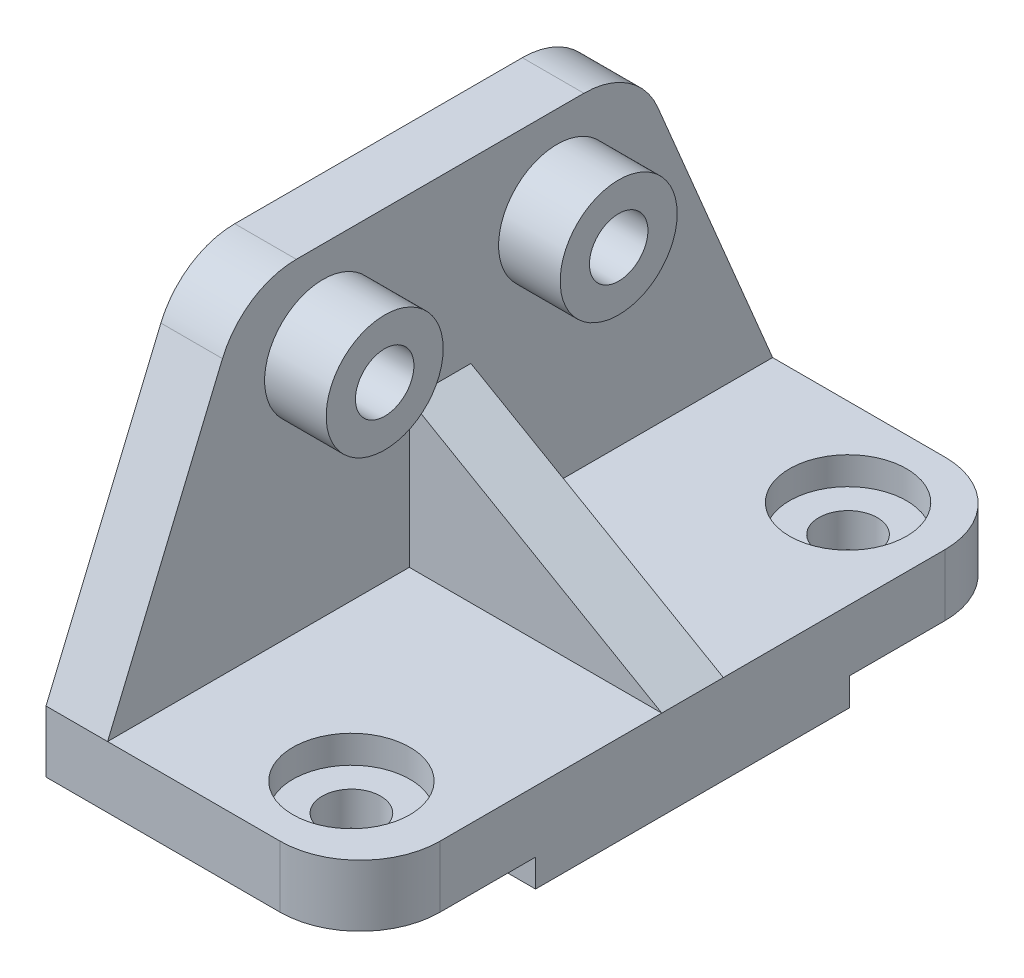
ISO-10303-21;
HEADER;
FILE_DESCRIPTION(('STEP AP214'),'2;1');
FILE_NAME('part.step','',(''),(''),'','','');
FILE_SCHEMA(('AUTOMOTIVE_DESIGN { 1 0 10303 214 1 1 1 1 }'));
ENDSEC;
DATA;
#1=APPLICATION_CONTEXT('core data for automotive mechanical design processes');
#2=APPLICATION_PROTOCOL_DEFINITION('international standard','automotive_design',2000,#1);
#3=PRODUCT_CONTEXT('',#1,'mechanical');
#4=PRODUCT('Part','Part','',(#3));
#5=PRODUCT_RELATED_PRODUCT_CATEGORY('part','',(#4));
#6=PRODUCT_DEFINITION_FORMATION('','',#4);
#7=PRODUCT_DEFINITION_CONTEXT('part definition',#1,'design');
#8=PRODUCT_DEFINITION('design','',#6,#7);
#9=PRODUCT_DEFINITION_SHAPE('','',#8);
#10=(LENGTH_UNIT() NAMED_UNIT(*) SI_UNIT(.MILLI.,.METRE.));
#11=(NAMED_UNIT(*) PLANE_ANGLE_UNIT() SI_UNIT($,.RADIAN.));
#12=(NAMED_UNIT(*) SI_UNIT($,.STERADIAN.) SOLID_ANGLE_UNIT());
#13=UNCERTAINTY_MEASURE_WITH_UNIT(LENGTH_MEASURE(1.E-05),#10,'distance_accuracy_value','');
#14=(GEOMETRIC_REPRESENTATION_CONTEXT(3) GLOBAL_UNCERTAINTY_ASSIGNED_CONTEXT((#13)) GLOBAL_UNIT_ASSIGNED_CONTEXT((#10,
#11,#12)) REPRESENTATION_CONTEXT('',''));
#15=CARTESIAN_POINT('',(0.,0.,0.));
#16=DIRECTION('',(0.,0.,1.));
#17=DIRECTION('',(1.,0.,0.));
#18=AXIS2_PLACEMENT_3D('',#15,#16,#17);
#19=CARTESIAN_POINT('',(102.,20.,-216.));
#20=DIRECTION('',(0.,-1.,0.));
#21=DIRECTION('',(0.,0.,-1.));
#22=AXIS2_PLACEMENT_3D('',#19,#20,#21);
#23=PLANE('',#22);
#24=CARTESIAN_POINT('',(73.,20.,-187.5));
#25=DIRECTION('',(0.,1.,0.));
#26=DIRECTION('',(0.,0.,1.));
#27=AXIS2_PLACEMENT_3D('',#24,#25,#26);
#28=CIRCLE('',#27,19.);
#29=CARTESIAN_POINT('',(73.,20.,-168.5));
#30=VERTEX_POINT('',#29);
#31=EDGE_CURVE('E246',#30,#30,#28,.T.);
#32=ORIENTED_EDGE('',*,*,#31,.F.);
#33=EDGE_LOOP('',(#32));
#34=FACE_BOUND('',#33,.T.);
#35=DIRECTION('',(-1.,0.,0.));
#36=VECTOR('',#35,1.);
#37=CARTESIAN_POINT('',(102.,20.,-118.));
#38=LINE('',#37,#36);
#39=CARTESIAN_POINT('',(102.,20.,-118.));
#40=VERTEX_POINT('',#39);
#41=CARTESIAN_POINT('',(20.,20.,-118.));
#42=VERTEX_POINT('',#41);
#43=EDGE_CURVE('E53',#40,#42,#38,.T.);
#44=ORIENTED_EDGE('',*,*,#43,.F.);
#45=DIRECTION('',(0.,0.,1.));
#46=VECTOR('',#45,1.);
#47=CARTESIAN_POINT('',(102.,20.,-216.));
#48=LINE('',#47,#46);
#49=CARTESIAN_POINT('',(102.,20.,-190.));
#50=VERTEX_POINT('',#49);
#51=EDGE_CURVE('E182',#50,#40,#48,.T.);
#52=ORIENTED_EDGE('',*,*,#51,.F.);
#53=CARTESIAN_POINT('',(76.,20.,-190.));
#54=DIRECTION('',(0.,-1.,0.));
#55=DIRECTION('',(0.,0.,-1.));
#56=AXIS2_PLACEMENT_3D('',#53,#54,#55);
#57=CIRCLE('',#56,26.);
#58=CARTESIAN_POINT('',(76.,20.,-216.));
#59=VERTEX_POINT('',#58);
#60=EDGE_CURVE('E280',#50,#59,#57,.F.);
#61=ORIENTED_EDGE('',*,*,#60,.T.);
#62=DIRECTION('',(-1.,0.,0.));
#63=VECTOR('',#62,1.);
#64=CARTESIAN_POINT('',(102.,20.,-216.));
#65=LINE('',#64,#63);
#66=CARTESIAN_POINT('',(20.,20.,-216.));
#67=VERTEX_POINT('',#66);
#68=EDGE_CURVE('E192',#59,#67,#65,.T.);
#69=ORIENTED_EDGE('',*,*,#68,.T.);
#70=DIRECTION('',(0.,0.,-1.));
#71=VECTOR('',#70,1.);
#72=CARTESIAN_POINT('',(20.,20.,0.));
#73=LINE('',#72,#71);
#74=EDGE_CURVE('E184',#42,#67,#73,.T.);
#75=ORIENTED_EDGE('',*,*,#74,.F.);
#76=EDGE_LOOP('',(#44,#52,#61,#69,#75));
#77=FACE_BOUND('',#76,.T.);
#78=ADVANCED_FACE('F39',(#34,#77),#23,.F.);
#79=CARTESIAN_POINT('',(70.69,20.,-28.5));
#80=DIRECTION('',(0.,1.,0.));
#81=DIRECTION('',(0.,0.,1.));
#82=AXIS2_PLACEMENT_3D('',#79,#80,#81);
#83=CIRCLE('',#82,19.);
#84=CARTESIAN_POINT('',(70.69,20.,-9.49999999999997));
#85=VERTEX_POINT('',#84);
#86=EDGE_CURVE('E252',#85,#85,#83,.T.);
#87=ORIENTED_EDGE('',*,*,#86,.F.);
#88=EDGE_LOOP('',(#87));
#89=FACE_BOUND('',#88,.T.);
#90=CARTESIAN_POINT('',(102.,20.,-98.));
#91=VERTEX_POINT('',#90);
#92=CARTESIAN_POINT('',(102.,20.,-26.));
#93=VERTEX_POINT('',#92);
#94=EDGE_CURVE('E195',#91,#93,#48,.T.);
#95=ORIENTED_EDGE('',*,*,#94,.F.);
#96=DIRECTION('',(-1.,0.,0.));
#97=VECTOR('',#96,1.);
#98=CARTESIAN_POINT('',(102.,20.,-98.));
#99=LINE('',#98,#97);
#100=CARTESIAN_POINT('',(20.,20.,-98.));
#101=VERTEX_POINT('',#100);
#102=EDGE_CURVE('E174',#91,#101,#99,.T.);
#103=ORIENTED_EDGE('',*,*,#102,.T.);
#104=CARTESIAN_POINT('',(20.,20.,0.));
#105=VERTEX_POINT('',#104);
#106=EDGE_CURVE('E296',#105,#101,#73,.T.);
#107=ORIENTED_EDGE('',*,*,#106,.F.);
#108=DIRECTION('',(-1.,0.,0.));
#109=VECTOR('',#108,1.);
#110=CARTESIAN_POINT('',(102.,20.,0.));
#111=LINE('',#110,#109);
#112=CARTESIAN_POINT('',(76.,20.,0.));
#113=VERTEX_POINT('',#112);
#114=EDGE_CURVE('E191',#113,#105,#111,.T.);
#115=ORIENTED_EDGE('',*,*,#114,.F.);
#116=CARTESIAN_POINT('',(76.,20.,-26.));
#117=DIRECTION('',(0.,-1.,0.));
#118=DIRECTION('',(0.,0.,-1.));
#119=AXIS2_PLACEMENT_3D('',#116,#117,#118);
#120=CIRCLE('',#119,26.);
#121=EDGE_CURVE('E273',#113,#93,#120,.F.);
#122=ORIENTED_EDGE('',*,*,#121,.T.);
#123=EDGE_LOOP('',(#95,#103,#107,#115,#122));
#124=FACE_BOUND('',#123,.T.);
#125=ADVANCED_FACE('F385',(#89,#124),#23,.F.);
#126=CARTESIAN_POINT('',(102.,20.,0.));
#127=DIRECTION('',(0.,0.,-1.));
#128=DIRECTION('',(-1.,0.,0.));
#129=AXIS2_PLACEMENT_3D('',#126,#127,#128);
#130=PLANE('',#129);
#131=DIRECTION('',(-1.,0.,0.));
#132=VECTOR('',#131,1.);
#133=CARTESIAN_POINT('',(102.,0.,0.));
#134=LINE('',#133,#132);
#135=CARTESIAN_POINT('',(76.,0.,0.));
#136=VERTEX_POINT('',#135);
#137=CARTESIAN_POINT('',(0.,0.,0.));
#138=VERTEX_POINT('',#137);
#139=EDGE_CURVE('E234',#136,#138,#134,.T.);
#140=ORIENTED_EDGE('',*,*,#139,.F.);
#141=DIRECTION('',(0.,-1.,0.));
#142=VECTOR('',#141,1.);
#143=CARTESIAN_POINT('',(76.,20.,0.));
#144=LINE('',#143,#142);
#145=EDGE_CURVE('E282',#136,#113,#144,.F.);
#146=ORIENTED_EDGE('',*,*,#145,.T.);
#147=ORIENTED_EDGE('',*,*,#114,.T.);
#148=DIRECTION('',(-1.,0.,0.));
#149=VECTOR('',#148,1.);
#150=CARTESIAN_POINT('',(20.,20.,0.));
#151=LINE('',#150,#149);
#152=CARTESIAN_POINT('',(0.,20.,0.));
#153=VERTEX_POINT('',#152);
#154=EDGE_CURVE('E203',#105,#153,#151,.T.);
#155=ORIENTED_EDGE('',*,*,#154,.T.);
#156=DIRECTION('',(0.,-1.,0.));
#157=VECTOR('',#156,1.);
#158=CARTESIAN_POINT('',(0.,20.,0.));
#159=LINE('',#158,#157);
#160=EDGE_CURVE('E202',#153,#138,#159,.T.);
#161=ORIENTED_EDGE('',*,*,#160,.T.);
#162=EDGE_LOOP('',(#140,#146,#147,#155,#161));
#163=FACE_BOUND('',#162,.T.);
#164=ADVANCED_FACE('F421',(#163),#130,.F.);
#165=CARTESIAN_POINT('',(102.,0.,0.));
#166=DIRECTION('',(0.,1.,0.));
#167=DIRECTION('',(0.,0.,1.));
#168=AXIS2_PLACEMENT_3D('',#165,#166,#167);
#169=PLANE('',#168);
#170=CARTESIAN_POINT('',(70.69,0.,-28.5));
#171=DIRECTION('',(0.,1.,0.));
#172=DIRECTION('',(0.,0.,1.));
#173=AXIS2_PLACEMENT_3D('',#170,#171,#172);
#174=CIRCLE('',#173,9.50000000000001);
#175=CARTESIAN_POINT('',(70.69,0.,-19.));
#176=VERTEX_POINT('',#175);
#177=EDGE_CURVE('E247',#176,#176,#174,.T.);
#178=ORIENTED_EDGE('',*,*,#177,.T.);
#179=EDGE_LOOP('',(#178));
#180=FACE_BOUND('',#179,.T.);
#181=DIRECTION('',(0.,0.,-1.));
#182=VECTOR('',#181,1.);
#183=CARTESIAN_POINT('',(102.,0.,0.));
#184=LINE('',#183,#182);
#185=CARTESIAN_POINT('',(102.,0.,-26.));
#186=VERTEX_POINT('',#185);
#187=CARTESIAN_POINT('',(102.,0.,-57.));
#188=VERTEX_POINT('',#187);
#189=EDGE_CURVE('E216',#186,#188,#184,.T.);
#190=ORIENTED_EDGE('',*,*,#189,.F.);
#191=CARTESIAN_POINT('',(76.,0.,-26.));
#192=DIRECTION('',(0.,1.,0.));
#193=DIRECTION('',(0.,0.,1.));
#194=AXIS2_PLACEMENT_3D('',#191,#192,#193);
#195=CIRCLE('',#194,26.);
#196=EDGE_CURVE('E61',#186,#136,#195,.F.);
#197=ORIENTED_EDGE('',*,*,#196,.T.);
#198=ORIENTED_EDGE('',*,*,#139,.T.);
#199=DIRECTION('',(0.,0.,-1.));
#200=VECTOR('',#199,1.);
#201=CARTESIAN_POINT('',(0.,0.,0.));
#202=LINE('',#201,#200);
#203=CARTESIAN_POINT('',(0.,0.,-57.));
#204=VERTEX_POINT('',#203);
#205=EDGE_CURVE('E201',#138,#204,#202,.T.);
#206=ORIENTED_EDGE('',*,*,#205,.T.);
#207=DIRECTION('',(-1.,0.,0.));
#208=VECTOR('',#207,1.);
#209=CARTESIAN_POINT('',(102.,0.,-57.));
#210=LINE('',#209,#208);
#211=EDGE_CURVE('E233',#188,#204,#210,.T.);
#212=ORIENTED_EDGE('',*,*,#211,.F.);
#213=EDGE_LOOP('',(#190,#197,#198,#206,#212));
#214=FACE_BOUND('',#213,.T.);
#215=ADVANCED_FACE('F386',(#180,#214),#169,.F.);
#216=CARTESIAN_POINT('',(102.,0.,-57.));
#217=DIRECTION('',(0.,0.,-1.));
#218=DIRECTION('',(-1.,0.,0.));
#219=AXIS2_PLACEMENT_3D('',#216,#217,#218);
#220=PLANE('',#219);
#221=DIRECTION('',(0.,-1.,0.));
#222=VECTOR('',#221,1.);
#223=CARTESIAN_POINT('',(0.,0.,-57.));
#224=LINE('',#223,#222);
#225=CARTESIAN_POINT('',(0.,-9.,-57.));
#226=VERTEX_POINT('',#225);
#227=EDGE_CURVE('E210',#204,#226,#224,.T.);
#228=ORIENTED_EDGE('',*,*,#227,.T.);
#229=DIRECTION('',(-1.,0.,0.));
#230=VECTOR('',#229,1.);
#231=CARTESIAN_POINT('',(102.,-9.,-57.));
#232=LINE('',#231,#230);
#233=CARTESIAN_POINT('',(102.,-9.,-57.));
#234=VERTEX_POINT('',#233);
#235=EDGE_CURVE('E226',#234,#226,#232,.T.);
#236=ORIENTED_EDGE('',*,*,#235,.F.);
#237=DIRECTION('',(0.,-1.,0.));
#238=VECTOR('',#237,1.);
#239=CARTESIAN_POINT('',(102.,0.,-57.));
#240=LINE('',#239,#238);
#241=EDGE_CURVE('E325',#188,#234,#240,.T.);
#242=ORIENTED_EDGE('',*,*,#241,.F.);
#243=ORIENTED_EDGE('',*,*,#211,.T.);
#244=EDGE_LOOP('',(#228,#236,#242,#243));
#245=FACE_BOUND('',#244,.T.);
#246=ADVANCED_FACE('F395',(#245),#220,.F.);
#247=CARTESIAN_POINT('',(102.,-9.,-57.));
#248=DIRECTION('',(0.,1.,0.));
#249=DIRECTION('',(0.,0.,1.));
#250=AXIS2_PLACEMENT_3D('',#247,#248,#249);
#251=PLANE('',#250);
#252=DIRECTION('',(0.,0.,-1.));
#253=VECTOR('',#252,1.);
#254=CARTESIAN_POINT('',(0.,-9.,-57.));
#255=LINE('',#254,#253);
#256=CARTESIAN_POINT('',(0.,-9.,-159.));
#257=VERTEX_POINT('',#256);
#258=EDGE_CURVE('E209',#226,#257,#255,.T.);
#259=ORIENTED_EDGE('',*,*,#258,.T.);
#260=DIRECTION('',(-1.,0.,0.));
#261=VECTOR('',#260,1.);
#262=CARTESIAN_POINT('',(102.,-9.,-159.));
#263=LINE('',#262,#261);
#264=CARTESIAN_POINT('',(102.,-9.,-159.));
#265=VERTEX_POINT('',#264);
#266=EDGE_CURVE('E223',#265,#257,#263,.T.);
#267=ORIENTED_EDGE('',*,*,#266,.F.);
#268=DIRECTION('',(0.,0.,-1.));
#269=VECTOR('',#268,1.);
#270=CARTESIAN_POINT('',(102.,-9.,-57.));
#271=LINE('',#270,#269);
#272=EDGE_CURVE('E322',#234,#265,#271,.T.);
#273=ORIENTED_EDGE('',*,*,#272,.F.);
#274=ORIENTED_EDGE('',*,*,#235,.T.);
#275=EDGE_LOOP('',(#259,#267,#273,#274));
#276=FACE_BOUND('',#275,.T.);
#277=ADVANCED_FACE('F399',(#276),#251,.F.);
#278=CARTESIAN_POINT('',(102.,-9.,-159.));
#279=DIRECTION('',(0.,0.,1.));
#280=DIRECTION('',(1.,0.,0.));
#281=AXIS2_PLACEMENT_3D('',#278,#279,#280);
#282=PLANE('',#281);
#283=DIRECTION('',(0.,1.,0.));
#284=VECTOR('',#283,1.);
#285=CARTESIAN_POINT('',(0.,-9.,-159.));
#286=LINE('',#285,#284);
#287=CARTESIAN_POINT('',(0.,0.,-159.));
#288=VERTEX_POINT('',#287);
#289=EDGE_CURVE('E214',#257,#288,#286,.T.);
#290=ORIENTED_EDGE('',*,*,#289,.T.);
#291=DIRECTION('',(-1.,0.,0.));
#292=VECTOR('',#291,1.);
#293=CARTESIAN_POINT('',(102.,0.,-159.));
#294=LINE('',#293,#292);
#295=CARTESIAN_POINT('',(102.,0.,-159.));
#296=VERTEX_POINT('',#295);
#297=EDGE_CURVE('E224',#296,#288,#294,.T.);
#298=ORIENTED_EDGE('',*,*,#297,.F.);
#299=DIRECTION('',(0.,1.,0.));
#300=VECTOR('',#299,1.);
#301=CARTESIAN_POINT('',(102.,-9.,-159.));
#302=LINE('',#301,#300);
#303=EDGE_CURVE('E329',#265,#296,#302,.T.);
#304=ORIENTED_EDGE('',*,*,#303,.F.);
#305=ORIENTED_EDGE('',*,*,#266,.T.);
#306=EDGE_LOOP('',(#290,#298,#304,#305));
#307=FACE_BOUND('',#306,.T.);
#308=ADVANCED_FACE('F402',(#307),#282,.F.);
#309=CARTESIAN_POINT('',(102.,0.,-159.));
#310=DIRECTION('',(0.,1.,0.));
#311=DIRECTION('',(0.,0.,1.));
#312=AXIS2_PLACEMENT_3D('',#309,#310,#311);
#313=PLANE('',#312);
#314=CARTESIAN_POINT('',(73.,0.,-187.5));
#315=DIRECTION('',(0.,1.,0.));
#316=DIRECTION('',(0.,0.,1.));
#317=AXIS2_PLACEMENT_3D('',#314,#315,#316);
#318=CIRCLE('',#317,9.5);
#319=CARTESIAN_POINT('',(73.,0.,-178.));
#320=VERTEX_POINT('',#319);
#321=EDGE_CURVE('E243',#320,#320,#318,.T.);
#322=ORIENTED_EDGE('',*,*,#321,.T.);
#323=EDGE_LOOP('',(#322));
#324=FACE_BOUND('',#323,.T.);
#325=DIRECTION('',(-1.,0.,0.));
#326=VECTOR('',#325,1.);
#327=CARTESIAN_POINT('',(102.,0.,-216.));
#328=LINE('',#327,#326);
#329=CARTESIAN_POINT('',(76.,0.,-216.));
#330=VERTEX_POINT('',#329);
#331=CARTESIAN_POINT('',(0.,0.,-216.));
#332=VERTEX_POINT('',#331);
#333=EDGE_CURVE('E217',#330,#332,#328,.T.);
#334=ORIENTED_EDGE('',*,*,#333,.F.);
#335=CARTESIAN_POINT('',(76.,0.,-190.));
#336=DIRECTION('',(0.,1.,0.));
#337=DIRECTION('',(0.,0.,1.));
#338=AXIS2_PLACEMENT_3D('',#335,#336,#337);
#339=CIRCLE('',#338,26.);
#340=CARTESIAN_POINT('',(102.,0.,-190.));
#341=VERTEX_POINT('',#340);
#342=EDGE_CURVE('E281',#330,#341,#339,.F.);
#343=ORIENTED_EDGE('',*,*,#342,.T.);
#344=DIRECTION('',(0.,0.,-1.));
#345=VECTOR('',#344,1.);
#346=CARTESIAN_POINT('',(102.,0.,-159.));
#347=LINE('',#346,#345);
#348=EDGE_CURVE('E196',#296,#341,#347,.T.);
#349=ORIENTED_EDGE('',*,*,#348,.F.);
#350=ORIENTED_EDGE('',*,*,#297,.T.);
#351=DIRECTION('',(0.,0.,-1.));
#352=VECTOR('',#351,1.);
#353=CARTESIAN_POINT('',(0.,0.,-159.));
#354=LINE('',#353,#352);
#355=EDGE_CURVE('E215',#288,#332,#354,.T.);
#356=ORIENTED_EDGE('',*,*,#355,.T.);
#357=EDGE_LOOP('',(#334,#343,#349,#350,#356));
#358=FACE_BOUND('',#357,.T.);
#359=ADVANCED_FACE('F401',(#324,#358),#313,.F.);
#360=CARTESIAN_POINT('',(102.,0.,-216.));
#361=DIRECTION('',(0.,0.,1.));
#362=DIRECTION('',(1.,0.,0.));
#363=AXIS2_PLACEMENT_3D('',#360,#361,#362);
#364=PLANE('',#363);
#365=ORIENTED_EDGE('',*,*,#68,.F.);
#366=DIRECTION('',(0.,1.,0.));
#367=VECTOR('',#366,1.);
#368=CARTESIAN_POINT('',(76.,0.,-216.));
#369=LINE('',#368,#367);
#370=EDGE_CURVE('E277',#59,#330,#369,.F.);
#371=ORIENTED_EDGE('',*,*,#370,.T.);
#372=ORIENTED_EDGE('',*,*,#333,.T.);
#373=DIRECTION('',(0.,1.,0.));
#374=VECTOR('',#373,1.);
#375=CARTESIAN_POINT('',(0.,0.,-216.));
#376=LINE('',#375,#374);
#377=CARTESIAN_POINT('',(0.,20.,-216.));
#378=VERTEX_POINT('',#377);
#379=EDGE_CURVE('E219',#332,#378,#376,.T.);
#380=ORIENTED_EDGE('',*,*,#379,.T.);
#381=DIRECTION('',(-1.,0.,0.));
#382=VECTOR('',#381,1.);
#383=CARTESIAN_POINT('',(20.,20.,-216.));
#384=LINE('',#383,#382);
#385=EDGE_CURVE('E302',#67,#378,#384,.T.);
#386=ORIENTED_EDGE('',*,*,#385,.F.);
#387=EDGE_LOOP('',(#365,#371,#372,#380,#386));
#388=FACE_BOUND('',#387,.T.);
#389=ADVANCED_FACE('F336',(#388),#364,.F.);
#390=CARTESIAN_POINT('',(102.,0.,0.));
#391=DIRECTION('',(1.,0.,0.));
#392=DIRECTION('',(0.,0.,-1.));
#393=AXIS2_PLACEMENT_3D('',#390,#391,#392);
#394=PLANE('',#393);
#395=ORIENTED_EDGE('',*,*,#272,.T.);
#396=ORIENTED_EDGE('',*,*,#303,.T.);
#397=ORIENTED_EDGE('',*,*,#348,.T.);
#398=DIRECTION('',(0.,1.,0.));
#399=VECTOR('',#398,1.);
#400=CARTESIAN_POINT('',(102.,20.,-190.));
#401=LINE('',#400,#399);
#402=EDGE_CURVE('E194',#341,#50,#401,.T.);
#403=ORIENTED_EDGE('',*,*,#402,.T.);
#404=ORIENTED_EDGE('',*,*,#51,.T.);
#405=DIRECTION('',(0.,0.,1.));
#406=VECTOR('',#405,1.);
#407=CARTESIAN_POINT('',(102.,20.,0.));
#408=LINE('',#407,#406);
#409=EDGE_CURVE('E164',#40,#91,#408,.T.);
#410=ORIENTED_EDGE('',*,*,#409,.T.);
#411=ORIENTED_EDGE('',*,*,#94,.T.);
#412=DIRECTION('',(0.,-1.,0.));
#413=VECTOR('',#412,1.);
#414=CARTESIAN_POINT('',(102.,0.,-26.));
#415=LINE('',#414,#413);
#416=EDGE_CURVE('E272',#93,#186,#415,.T.);
#417=ORIENTED_EDGE('',*,*,#416,.T.);
#418=ORIENTED_EDGE('',*,*,#189,.T.);
#419=ORIENTED_EDGE('',*,*,#241,.T.);
#420=EDGE_LOOP('',(#395,#396,#397,#403,#404,#410,#411,#417,#418,#419));
#421=FACE_BOUND('',#420,.T.);
#422=ADVANCED_FACE('F189',(#421),#394,.T.);
#423=CARTESIAN_POINT('',(0.,0.,0.));
#424=DIRECTION('',(1.,0.,0.));
#425=DIRECTION('',(0.,0.,-1.));
#426=AXIS2_PLACEMENT_3D('',#423,#424,#425);
#427=PLANE('',#426);
#428=ORIENTED_EDGE('',*,*,#289,.F.);
#429=ORIENTED_EDGE('',*,*,#258,.F.);
#430=ORIENTED_EDGE('',*,*,#227,.F.);
#431=ORIENTED_EDGE('',*,*,#205,.F.);
#432=ORIENTED_EDGE('',*,*,#160,.F.);
#433=DIRECTION('',(0.,-0.922295402517783,0.386485692483642));
#434=VECTOR('',#433,1.);
#435=CARTESIAN_POINT('',(0.,125.,-44.));
#436=LINE('',#435,#434);
#437=CARTESIAN_POINT('',(0.,109.048628004575,-37.3156155447742));
#438=VERTEX_POINT('',#437);
#439=EDGE_CURVE('E320',#438,#153,#436,.T.);
#440=ORIENTED_EDGE('',*,*,#439,.F.);
#441=CARTESIAN_POINT('',(0.,99.,-61.2952960102365));
#442=DIRECTION('',(1.,0.,0.));
#443=DIRECTION('',(0.,0.,-1.));
#444=AXIS2_PLACEMENT_3D('',#441,#442,#443);
#445=CIRCLE('',#444,26.);
#446=CARTESIAN_POINT('',(0.,125.,-61.2952960102365));
#447=VERTEX_POINT('',#446);
#448=EDGE_CURVE('E251',#438,#447,#445,.F.);
#449=ORIENTED_EDGE('',*,*,#448,.T.);
#450=DIRECTION('',(0.,0.,1.));
#451=VECTOR('',#450,1.);
#452=CARTESIAN_POINT('',(0.,125.,-44.));
#453=LINE('',#452,#451);
#454=CARTESIAN_POINT('',(0.,125.,-154.704703989763));
#455=VERTEX_POINT('',#454);
#456=EDGE_CURVE('E313',#455,#447,#453,.T.);
#457=ORIENTED_EDGE('',*,*,#456,.F.);
#458=CARTESIAN_POINT('',(0.,99.,-154.704703989763));
#459=DIRECTION('',(1.,0.,0.));
#460=DIRECTION('',(0.,0.,-1.));
#461=AXIS2_PLACEMENT_3D('',#458,#459,#460);
#462=CIRCLE('',#461,26.);
#463=CARTESIAN_POINT('',(0.,109.048628004575,-178.684384455226));
#464=VERTEX_POINT('',#463);
#465=EDGE_CURVE('E262',#455,#464,#462,.F.);
#466=ORIENTED_EDGE('',*,*,#465,.T.);
#467=DIRECTION('',(0.,0.922295402517783,0.386485692483642));
#468=VECTOR('',#467,1.);
#469=CARTESIAN_POINT('',(0.,125.,-172.));
#470=LINE('',#469,#468);
#471=EDGE_CURVE('E311',#378,#464,#470,.T.);
#472=ORIENTED_EDGE('',*,*,#471,.F.);
#473=ORIENTED_EDGE('',*,*,#379,.F.);
#474=ORIENTED_EDGE('',*,*,#355,.F.);
#475=EDGE_LOOP('',(#428,#429,#430,#431,#432,#440,#449,#457,#466,#472,#473,#474));
#476=FACE_BOUND('',#475,.T.);
#477=ADVANCED_FACE('F403',(#476),#427,.F.);
#478=CARTESIAN_POINT('',(20.,125.,-172.));
#479=DIRECTION('',(0.,-0.386485692483642,0.922295402517783));
#480=DIRECTION('',(0.,-0.922295402517783,-0.386485692483642));
#481=AXIS2_PLACEMENT_3D('',#478,#479,#480);
#482=PLANE('',#481);
#483=ORIENTED_EDGE('',*,*,#471,.T.);
#484=DIRECTION('',(-1.,0.,0.));
#485=VECTOR('',#484,1.);
#486=CARTESIAN_POINT('',(20.,109.048628004575,-178.684384455226));
#487=LINE('',#486,#485);
#488=CARTESIAN_POINT('',(20.,109.048628004575,-178.684384455226));
#489=VERTEX_POINT('',#488);
#490=EDGE_CURVE('E269',#464,#489,#487,.F.);
#491=ORIENTED_EDGE('',*,*,#490,.T.);
#492=DIRECTION('',(0.,0.922295402517783,0.386485692483642));
#493=VECTOR('',#492,1.);
#494=CARTESIAN_POINT('',(20.,125.,-172.));
#495=LINE('',#494,#493);
#496=EDGE_CURVE('E319',#67,#489,#495,.T.);
#497=ORIENTED_EDGE('',*,*,#496,.F.);
#498=ORIENTED_EDGE('',*,*,#385,.T.);
#499=EDGE_LOOP('',(#483,#491,#497,#498));
#500=FACE_BOUND('',#499,.T.);
#501=ADVANCED_FACE('F342',(#500),#482,.F.);
#502=CARTESIAN_POINT('',(20.,125.,-44.));
#503=DIRECTION('',(0.,-1.,0.));
#504=DIRECTION('',(0.,0.,-1.));
#505=AXIS2_PLACEMENT_3D('',#502,#503,#504);
#506=PLANE('',#505);
#507=DIRECTION('',(0.,0.,1.));
#508=VECTOR('',#507,1.);
#509=CARTESIAN_POINT('',(20.,125.,-44.));
#510=LINE('',#509,#508);
#511=CARTESIAN_POINT('',(20.,125.,-154.704703989763));
#512=VERTEX_POINT('',#511);
#513=CARTESIAN_POINT('',(20.,125.,-61.2952960102365));
#514=VERTEX_POINT('',#513);
#515=EDGE_CURVE('E350',#512,#514,#510,.T.);
#516=ORIENTED_EDGE('',*,*,#515,.F.);
#517=DIRECTION('',(-1.,0.,0.));
#518=VECTOR('',#517,1.);
#519=CARTESIAN_POINT('',(20.,125.,-154.704703989763));
#520=LINE('',#519,#518);
#521=EDGE_CURVE('E261',#512,#455,#520,.T.);
#522=ORIENTED_EDGE('',*,*,#521,.T.);
#523=ORIENTED_EDGE('',*,*,#456,.T.);
#524=DIRECTION('',(-1.,0.,0.));
#525=VECTOR('',#524,1.);
#526=CARTESIAN_POINT('',(20.,125.,-61.2952960102365));
#527=LINE('',#526,#525);
#528=EDGE_CURVE('E256',#447,#514,#527,.F.);
#529=ORIENTED_EDGE('',*,*,#528,.T.);
#530=EDGE_LOOP('',(#516,#522,#523,#529));
#531=FACE_BOUND('',#530,.T.);
#532=ADVANCED_FACE('F411',(#531),#506,.F.);
#533=CARTESIAN_POINT('',(20.,125.,-44.));
#534=DIRECTION('',(0.,-0.386485692483642,-0.922295402517783));
#535=DIRECTION('',(0.,0.922295402517783,-0.386485692483642));
#536=AXIS2_PLACEMENT_3D('',#533,#534,#535);
#537=PLANE('',#536);
#538=DIRECTION('',(0.,-0.922295402517783,0.386485692483642));
#539=VECTOR('',#538,1.);
#540=CARTESIAN_POINT('',(20.,125.,-44.));
#541=LINE('',#540,#539);
#542=CARTESIAN_POINT('',(20.,109.048628004575,-37.3156155447742));
#543=VERTEX_POINT('',#542);
#544=EDGE_CURVE('E297',#543,#105,#541,.T.);
#545=ORIENTED_EDGE('',*,*,#544,.F.);
#546=DIRECTION('',(-1.,0.,0.));
#547=VECTOR('',#546,1.);
#548=CARTESIAN_POINT('',(20.,109.048628004575,-37.3156155447742));
#549=LINE('',#548,#547);
#550=EDGE_CURVE('E245',#543,#438,#549,.T.);
#551=ORIENTED_EDGE('',*,*,#550,.T.);
#552=ORIENTED_EDGE('',*,*,#439,.T.);
#553=ORIENTED_EDGE('',*,*,#154,.F.);
#554=EDGE_LOOP('',(#545,#551,#552,#553));
#555=FACE_BOUND('',#554,.T.);
#556=ADVANCED_FACE('F416',(#555),#537,.F.);
#557=CARTESIAN_POINT('',(20.,0.,0.));
#558=DIRECTION('',(1.,0.,0.));
#559=DIRECTION('',(0.,0.,-1.));
#560=AXIS2_PLACEMENT_3D('',#557,#558,#559);
#561=PLANE('',#560);
#562=DIRECTION('',(0.,-1.,0.));
#563=VECTOR('',#562,1.);
#564=CARTESIAN_POINT('',(20.,0.,-98.));
#565=LINE('',#564,#563);
#566=CARTESIAN_POINT('',(20.,67.3427220735494,-98.));
#567=VERTEX_POINT('',#566);
#568=EDGE_CURVE('E11',#567,#101,#565,.T.);
#569=ORIENTED_EDGE('',*,*,#568,.F.);
#570=DIRECTION('',(0.,0.,1.));
#571=VECTOR('',#570,1.);
#572=CARTESIAN_POINT('',(20.,67.3427220735494,0.));
#573=LINE('',#572,#571);
#574=CARTESIAN_POINT('',(20.,67.3427220735494,-118.));
#575=VERTEX_POINT('',#574);
#576=EDGE_CURVE('E50',#575,#567,#573,.T.);
#577=ORIENTED_EDGE('',*,*,#576,.F.);
#578=DIRECTION('',(0.,-1.,0.));
#579=VECTOR('',#578,1.);
#580=CARTESIAN_POINT('',(20.,0.,-118.));
#581=LINE('',#580,#579);
#582=EDGE_CURVE('E178',#575,#42,#581,.T.);
#583=ORIENTED_EDGE('',*,*,#582,.T.);
#584=ORIENTED_EDGE('',*,*,#74,.T.);
#585=ORIENTED_EDGE('',*,*,#496,.T.);
#586=CARTESIAN_POINT('',(20.,99.,-154.704703989763));
#587=DIRECTION('',(1.,0.,0.));
#588=DIRECTION('',(0.,0.,-1.));
#589=AXIS2_PLACEMENT_3D('',#586,#587,#588);
#590=CIRCLE('',#589,26.);
#591=EDGE_CURVE('E266',#489,#512,#590,.T.);
#592=ORIENTED_EDGE('',*,*,#591,.T.);
#593=ORIENTED_EDGE('',*,*,#515,.T.);
#594=CARTESIAN_POINT('',(20.,99.,-61.2952960102365));
#595=DIRECTION('',(1.,0.,0.));
#596=DIRECTION('',(0.,0.,-1.));
#597=AXIS2_PLACEMENT_3D('',#594,#595,#596);
#598=CIRCLE('',#597,26.);
#599=EDGE_CURVE('E257',#514,#543,#598,.T.);
#600=ORIENTED_EDGE('',*,*,#599,.T.);
#601=ORIENTED_EDGE('',*,*,#544,.T.);
#602=ORIENTED_EDGE('',*,*,#106,.T.);
#603=EDGE_LOOP('',(#569,#577,#583,#584,#585,#592,#593,#600,#601,#602));
#604=FACE_BOUND('',#603,.T.);
#605=CARTESIAN_POINT('',(20.,96.,-146.));
#606=DIRECTION('',(1.,0.,0.));
#607=DIRECTION('',(0.,0.,-1.));
#608=AXIS2_PLACEMENT_3D('',#605,#606,#607);
#609=CIRCLE('',#608,19.);
#610=CARTESIAN_POINT('',(20.,96.,-165.));
#611=VERTEX_POINT('',#610);
#612=EDGE_CURVE('E359',#611,#611,#609,.T.);
#613=ORIENTED_EDGE('',*,*,#612,.F.);
#614=EDGE_LOOP('',(#613));
#615=FACE_BOUND('',#614,.T.);
#616=CARTESIAN_POINT('',(20.,96.,-70.));
#617=DIRECTION('',(1.,0.,0.));
#618=DIRECTION('',(0.,0.,-1.));
#619=AXIS2_PLACEMENT_3D('',#616,#617,#618);
#620=CIRCLE('',#619,19.);
#621=CARTESIAN_POINT('',(20.,96.,-89.));
#622=VERTEX_POINT('',#621);
#623=EDGE_CURVE('E352',#622,#622,#620,.T.);
#624=ORIENTED_EDGE('',*,*,#623,.F.);
#625=EDGE_LOOP('',(#624));
#626=FACE_BOUND('',#625,.T.);
#627=ADVANCED_FACE('F295',(#604,#615,#626),#561,.T.);
#628=CARTESIAN_POINT('',(40.,96.,-70.));
#629=DIRECTION('',(1.,0.,0.));
#630=DIRECTION('',(0.,0.,-1.));
#631=AXIS2_PLACEMENT_3D('',#628,#629,#630);
#632=PLANE('',#631);
#633=CARTESIAN_POINT('',(40.,96.,-70.));
#634=DIRECTION('',(1.,0.,0.));
#635=DIRECTION('',(0.,0.,-1.));
#636=AXIS2_PLACEMENT_3D('',#633,#634,#635);
#637=CIRCLE('',#636,19.);
#638=CARTESIAN_POINT('',(40.,96.,-89.));
#639=VERTEX_POINT('',#638);
#640=EDGE_CURVE('E314',#639,#639,#637,.T.);
#641=ORIENTED_EDGE('',*,*,#640,.T.);
#642=EDGE_LOOP('',(#641));
#643=FACE_BOUND('',#642,.T.);
#644=CARTESIAN_POINT('',(40.,96.,-70.));
#645=DIRECTION('',(1.,0.,0.));
#646=DIRECTION('',(0.,0.,-1.));
#647=AXIS2_PLACEMENT_3D('',#644,#645,#646);
#648=CIRCLE('',#647,9.49999999999999);
#649=CARTESIAN_POINT('',(40.,96.,-79.5));
#650=VERTEX_POINT('',#649);
#651=EDGE_CURVE('E351',#650,#650,#648,.T.);
#652=ORIENTED_EDGE('',*,*,#651,.F.);
#653=EDGE_LOOP('',(#652));
#654=FACE_BOUND('',#653,.T.);
#655=ADVANCED_FACE('F574',(#643,#654),#632,.T.);
#656=CARTESIAN_POINT('',(40.,96.,-70.));
#657=DIRECTION('',(-1.,0.,0.));
#658=DIRECTION('',(0.,0.,1.));
#659=AXIS2_PLACEMENT_3D('',#656,#657,#658);
#660=CYLINDRICAL_SURFACE('',#659,19.);
#661=ORIENTED_EDGE('',*,*,#640,.F.);
#662=EDGE_LOOP('',(#661));
#663=FACE_BOUND('',#662,.T.);
#664=ORIENTED_EDGE('',*,*,#623,.T.);
#665=EDGE_LOOP('',(#664));
#666=FACE_BOUND('',#665,.T.);
#667=ADVANCED_FACE('F572',(#663,#666),#660,.T.);
#668=CARTESIAN_POINT('',(40.,96.,-70.));
#669=DIRECTION('',(-1.,0.,0.));
#670=DIRECTION('',(0.,0.,1.));
#671=AXIS2_PLACEMENT_3D('',#668,#669,#670);
#672=CYLINDRICAL_SURFACE('',#671,9.49999999999999);
#673=ORIENTED_EDGE('',*,*,#651,.T.);
#674=EDGE_LOOP('',(#673));
#675=FACE_BOUND('',#674,.T.);
#676=CARTESIAN_POINT('',(20.,96.,-70.));
#677=DIRECTION('',(1.,0.,0.));
#678=DIRECTION('',(0.,0.,-1.));
#679=AXIS2_PLACEMENT_3D('',#676,#677,#678);
#680=CIRCLE('',#679,9.49999999999999);
#681=CARTESIAN_POINT('',(20.,96.,-79.5));
#682=VERTEX_POINT('',#681);
#683=EDGE_CURVE('E236',#682,#682,#680,.F.);
#684=ORIENTED_EDGE('',*,*,#683,.T.);
#685=EDGE_LOOP('',(#684));
#686=FACE_BOUND('',#685,.T.);
#687=ADVANCED_FACE('F569',(#675,#686),#672,.F.);
#688=ORIENTED_EDGE('',*,*,#683,.F.);
#689=EDGE_LOOP('',(#688));
#690=FACE_BOUND('',#689,.T.);
#691=ADVANCED_FACE('F564',(#690),#561,.T.);
#692=CARTESIAN_POINT('',(40.,96.,-146.));
#693=DIRECTION('',(1.,0.,0.));
#694=DIRECTION('',(0.,0.,-1.));
#695=AXIS2_PLACEMENT_3D('',#692,#693,#694);
#696=PLANE('',#695);
#697=CARTESIAN_POINT('',(40.,96.,-146.));
#698=DIRECTION('',(1.,0.,0.));
#699=DIRECTION('',(0.,0.,-1.));
#700=AXIS2_PLACEMENT_3D('',#697,#698,#699);
#701=CIRCLE('',#700,19.);
#702=CARTESIAN_POINT('',(40.,96.,-165.));
#703=VERTEX_POINT('',#702);
#704=EDGE_CURVE('E360',#703,#703,#701,.T.);
#705=ORIENTED_EDGE('',*,*,#704,.T.);
#706=EDGE_LOOP('',(#705));
#707=FACE_BOUND('',#706,.T.);
#708=CARTESIAN_POINT('',(40.,96.,-146.));
#709=DIRECTION('',(1.,0.,0.));
#710=DIRECTION('',(0.,0.,-1.));
#711=AXIS2_PLACEMENT_3D('',#708,#709,#710);
#712=CIRCLE('',#711,9.49999999999998);
#713=CARTESIAN_POINT('',(40.,96.,-155.5));
#714=VERTEX_POINT('',#713);
#715=EDGE_CURVE('E361',#714,#714,#712,.T.);
#716=ORIENTED_EDGE('',*,*,#715,.F.);
#717=EDGE_LOOP('',(#716));
#718=FACE_BOUND('',#717,.T.);
#719=ADVANCED_FACE('F565',(#707,#718),#696,.T.);
#720=CARTESIAN_POINT('',(40.,96.,-146.));
#721=DIRECTION('',(-1.,0.,0.));
#722=DIRECTION('',(0.,0.,1.));
#723=AXIS2_PLACEMENT_3D('',#720,#721,#722);
#724=CYLINDRICAL_SURFACE('',#723,19.);
#725=ORIENTED_EDGE('',*,*,#704,.F.);
#726=EDGE_LOOP('',(#725));
#727=FACE_BOUND('',#726,.T.);
#728=ORIENTED_EDGE('',*,*,#612,.T.);
#729=EDGE_LOOP('',(#728));
#730=FACE_BOUND('',#729,.T.);
#731=ADVANCED_FACE('F557',(#727,#730),#724,.T.);
#732=CARTESIAN_POINT('',(40.,96.,-146.));
#733=DIRECTION('',(-1.,0.,0.));
#734=DIRECTION('',(0.,0.,1.));
#735=AXIS2_PLACEMENT_3D('',#732,#733,#734);
#736=CYLINDRICAL_SURFACE('',#735,9.49999999999998);
#737=ORIENTED_EDGE('',*,*,#715,.T.);
#738=EDGE_LOOP('',(#737));
#739=FACE_BOUND('',#738,.T.);
#740=CARTESIAN_POINT('',(20.,96.,-146.));
#741=DIRECTION('',(1.,0.,0.));
#742=DIRECTION('',(0.,0.,-1.));
#743=AXIS2_PLACEMENT_3D('',#740,#741,#742);
#744=CIRCLE('',#743,9.49999999999998);
#745=CARTESIAN_POINT('',(20.,96.,-155.5));
#746=VERTEX_POINT('',#745);
#747=EDGE_CURVE('E237',#746,#746,#744,.F.);
#748=ORIENTED_EDGE('',*,*,#747,.T.);
#749=EDGE_LOOP('',(#748));
#750=FACE_BOUND('',#749,.T.);
#751=ADVANCED_FACE('F560',(#739,#750),#736,.F.);
#752=ORIENTED_EDGE('',*,*,#747,.F.);
#753=EDGE_LOOP('',(#752));
#754=FACE_BOUND('',#753,.T.);
#755=ADVANCED_FACE('F554',(#754),#561,.T.);
#756=CARTESIAN_POINT('',(73.,11.,-187.5));
#757=DIRECTION('',(0.,1.,0.));
#758=DIRECTION('',(0.,0.,1.));
#759=AXIS2_PLACEMENT_3D('',#756,#757,#758);
#760=CYLINDRICAL_SURFACE('',#759,19.);
#761=CARTESIAN_POINT('',(73.,11.,-187.5));
#762=DIRECTION('',(0.,1.,0.));
#763=DIRECTION('',(0.,0.,1.));
#764=AXIS2_PLACEMENT_3D('',#761,#762,#763);
#765=CIRCLE('',#764,19.);
#766=CARTESIAN_POINT('',(73.,11.,-168.5));
#767=VERTEX_POINT('',#766);
#768=EDGE_CURVE('E368',#767,#767,#765,.T.);
#769=ORIENTED_EDGE('',*,*,#768,.F.);
#770=EDGE_LOOP('',(#769));
#771=FACE_BOUND('',#770,.T.);
#772=ORIENTED_EDGE('',*,*,#31,.T.);
#773=EDGE_LOOP('',(#772));
#774=FACE_BOUND('',#773,.T.);
#775=ADVANCED_FACE('F553',(#771,#774),#760,.F.);
#776=CARTESIAN_POINT('',(73.,11.,-187.5));
#777=DIRECTION('',(0.,1.,0.));
#778=DIRECTION('',(0.,0.,1.));
#779=AXIS2_PLACEMENT_3D('',#776,#777,#778);
#780=PLANE('',#779);
#781=CARTESIAN_POINT('',(73.,11.,-187.5));
#782=DIRECTION('',(0.,1.,0.));
#783=DIRECTION('',(0.,0.,1.));
#784=AXIS2_PLACEMENT_3D('',#781,#782,#783);
#785=CIRCLE('',#784,9.5);
#786=CARTESIAN_POINT('',(73.,11.,-178.));
#787=VERTEX_POINT('',#786);
#788=EDGE_CURVE('E250',#787,#787,#785,.T.);
#789=ORIENTED_EDGE('',*,*,#788,.F.);
#790=EDGE_LOOP('',(#789));
#791=FACE_BOUND('',#790,.T.);
#792=ORIENTED_EDGE('',*,*,#768,.T.);
#793=EDGE_LOOP('',(#792));
#794=FACE_BOUND('',#793,.T.);
#795=ADVANCED_FACE('F549',(#791,#794),#780,.T.);
#796=CARTESIAN_POINT('',(73.,-9.,-187.5));
#797=DIRECTION('',(0.,1.,0.));
#798=DIRECTION('',(0.,0.,1.));
#799=AXIS2_PLACEMENT_3D('',#796,#797,#798);
#800=CYLINDRICAL_SURFACE('',#799,9.5);
#801=ORIENTED_EDGE('',*,*,#788,.T.);
#802=EDGE_LOOP('',(#801));
#803=FACE_BOUND('',#802,.T.);
#804=ORIENTED_EDGE('',*,*,#321,.F.);
#805=EDGE_LOOP('',(#804));
#806=FACE_BOUND('',#805,.T.);
#807=ADVANCED_FACE('F545',(#803,#806),#800,.F.);
#808=CARTESIAN_POINT('',(70.69,11.,-28.5));
#809=DIRECTION('',(0.,1.,0.));
#810=DIRECTION('',(0.,0.,1.));
#811=AXIS2_PLACEMENT_3D('',#808,#809,#810);
#812=CYLINDRICAL_SURFACE('',#811,19.);
#813=CARTESIAN_POINT('',(70.69,11.,-28.5));
#814=DIRECTION('',(0.,1.,0.));
#815=DIRECTION('',(0.,0.,1.));
#816=AXIS2_PLACEMENT_3D('',#813,#814,#815);
#817=CIRCLE('',#816,19.);
#818=CARTESIAN_POINT('',(70.69,11.,-9.49999999999997));
#819=VERTEX_POINT('',#818);
#820=EDGE_CURVE('E374',#819,#819,#817,.T.);
#821=ORIENTED_EDGE('',*,*,#820,.F.);
#822=EDGE_LOOP('',(#821));
#823=FACE_BOUND('',#822,.T.);
#824=ORIENTED_EDGE('',*,*,#86,.T.);
#825=EDGE_LOOP('',(#824));
#826=FACE_BOUND('',#825,.T.);
#827=ADVANCED_FACE('F538',(#823,#826),#812,.F.);
#828=CARTESIAN_POINT('',(70.69,11.,-28.5));
#829=DIRECTION('',(0.,1.,0.));
#830=DIRECTION('',(0.,0.,1.));
#831=AXIS2_PLACEMENT_3D('',#828,#829,#830);
#832=PLANE('',#831);
#833=CARTESIAN_POINT('',(70.69,11.,-28.5));
#834=DIRECTION('',(0.,1.,0.));
#835=DIRECTION('',(0.,0.,1.));
#836=AXIS2_PLACEMENT_3D('',#833,#834,#835);
#837=CIRCLE('',#836,9.50000000000001);
#838=CARTESIAN_POINT('',(70.69,11.,-19.));
#839=VERTEX_POINT('',#838);
#840=EDGE_CURVE('E172',#839,#839,#837,.T.);
#841=ORIENTED_EDGE('',*,*,#840,.F.);
#842=EDGE_LOOP('',(#841));
#843=FACE_BOUND('',#842,.T.);
#844=ORIENTED_EDGE('',*,*,#820,.T.);
#845=EDGE_LOOP('',(#844));
#846=FACE_BOUND('',#845,.T.);
#847=ADVANCED_FACE('F533',(#843,#846),#832,.T.);
#848=CARTESIAN_POINT('',(70.69,-9.,-28.5));
#849=DIRECTION('',(0.,1.,0.));
#850=DIRECTION('',(0.,0.,1.));
#851=AXIS2_PLACEMENT_3D('',#848,#849,#850);
#852=CYLINDRICAL_SURFACE('',#851,9.50000000000001);
#853=ORIENTED_EDGE('',*,*,#840,.T.);
#854=EDGE_LOOP('',(#853));
#855=FACE_BOUND('',#854,.T.);
#856=ORIENTED_EDGE('',*,*,#177,.F.);
#857=EDGE_LOOP('',(#856));
#858=FACE_BOUND('',#857,.T.);
#859=ADVANCED_FACE('F457',(#855,#858),#852,.F.);
#860=CARTESIAN_POINT('',(20.,99.,-61.2952960102365));
#861=DIRECTION('',(-1.,0.,0.));
#862=DIRECTION('',(0.,0.,1.));
#863=AXIS2_PLACEMENT_3D('',#860,#861,#862);
#864=CYLINDRICAL_SURFACE('',#863,26.);
#865=ORIENTED_EDGE('',*,*,#599,.F.);
#866=ORIENTED_EDGE('',*,*,#528,.F.);
#867=ORIENTED_EDGE('',*,*,#448,.F.);
#868=ORIENTED_EDGE('',*,*,#550,.F.);
#869=EDGE_LOOP('',(#865,#866,#867,#868));
#870=FACE_BOUND('',#869,.T.);
#871=ADVANCED_FACE('F419',(#870),#864,.T.);
#872=CARTESIAN_POINT('',(20.,99.,-154.704703989763));
#873=DIRECTION('',(-1.,0.,0.));
#874=DIRECTION('',(0.,0.,1.));
#875=AXIS2_PLACEMENT_3D('',#872,#873,#874);
#876=CYLINDRICAL_SURFACE('',#875,26.);
#877=ORIENTED_EDGE('',*,*,#591,.F.);
#878=ORIENTED_EDGE('',*,*,#490,.F.);
#879=ORIENTED_EDGE('',*,*,#465,.F.);
#880=ORIENTED_EDGE('',*,*,#521,.F.);
#881=EDGE_LOOP('',(#877,#878,#879,#880));
#882=FACE_BOUND('',#881,.T.);
#883=ADVANCED_FACE('F410',(#882),#876,.T.);
#884=CARTESIAN_POINT('',(76.,0.,-190.));
#885=DIRECTION('',(0.,-1.,0.));
#886=DIRECTION('',(0.,0.,-1.));
#887=AXIS2_PLACEMENT_3D('',#884,#885,#886);
#888=CYLINDRICAL_SURFACE('',#887,26.);
#889=ORIENTED_EDGE('',*,*,#342,.F.);
#890=ORIENTED_EDGE('',*,*,#370,.F.);
#891=ORIENTED_EDGE('',*,*,#60,.F.);
#892=ORIENTED_EDGE('',*,*,#402,.F.);
#893=EDGE_LOOP('',(#889,#890,#891,#892));
#894=FACE_BOUND('',#893,.T.);
#895=ADVANCED_FACE('F335',(#894),#888,.T.);
#896=CARTESIAN_POINT('',(76.,0.,-26.));
#897=DIRECTION('',(0.,1.,0.));
#898=DIRECTION('',(0.,0.,1.));
#899=AXIS2_PLACEMENT_3D('',#896,#897,#898);
#900=CYLINDRICAL_SURFACE('',#899,26.);
#901=ORIENTED_EDGE('',*,*,#121,.F.);
#902=ORIENTED_EDGE('',*,*,#145,.F.);
#903=ORIENTED_EDGE('',*,*,#196,.F.);
#904=ORIENTED_EDGE('',*,*,#416,.F.);
#905=EDGE_LOOP('',(#901,#902,#903,#904));
#906=FACE_BOUND('',#905,.T.);
#907=ADVANCED_FACE('F41',(#906),#900,.T.);
#908=CARTESIAN_POINT('',(102.,20.,-108.));
#909=DIRECTION('',(0.500000000000001,0.866025403784438,0.));
#910=DIRECTION('',(-0.866025403784438,0.500000000000001,0.));
#911=AXIS2_PLACEMENT_3D('',#908,#909,#910);
#912=PLANE('',#911);
#913=ORIENTED_EDGE('',*,*,#409,.F.);
#914=DIRECTION('',(-0.866025403784438,0.500000000000001,0.));
#915=VECTOR('',#914,1.);
#916=CARTESIAN_POINT('',(102.,20.,-118.));
#917=LINE('',#916,#915);
#918=EDGE_CURVE('E170',#40,#575,#917,.T.);
#919=ORIENTED_EDGE('',*,*,#918,.T.);
#920=ORIENTED_EDGE('',*,*,#576,.T.);
#921=DIRECTION('',(-0.866025403784438,0.500000000000001,0.));
#922=VECTOR('',#921,1.);
#923=CARTESIAN_POINT('',(102.,20.,-98.));
#924=LINE('',#923,#922);
#925=EDGE_CURVE('E167',#91,#567,#924,.T.);
#926=ORIENTED_EDGE('',*,*,#925,.F.);
#927=EDGE_LOOP('',(#913,#919,#920,#926));
#928=FACE_BOUND('',#927,.T.);
#929=ADVANCED_FACE('F168',(#928),#912,.T.);
#930=CARTESIAN_POINT('',(51.,58.,-98.));
#931=DIRECTION('',(0.,0.,1.));
#932=DIRECTION('',(1.,0.,0.));
#933=AXIS2_PLACEMENT_3D('',#930,#931,#932);
#934=PLANE('',#933);
#935=ORIENTED_EDGE('',*,*,#102,.F.);
#936=ORIENTED_EDGE('',*,*,#925,.T.);
#937=ORIENTED_EDGE('',*,*,#568,.T.);
#938=EDGE_LOOP('',(#935,#936,#937));
#939=FACE_BOUND('',#938,.T.);
#940=ADVANCED_FACE('F288',(#939),#934,.T.);
#941=CARTESIAN_POINT('',(51.,58.,-118.));
#942=DIRECTION('',(0.,0.,1.));
#943=DIRECTION('',(1.,0.,0.));
#944=AXIS2_PLACEMENT_3D('',#941,#942,#943);
#945=PLANE('',#944);
#946=ORIENTED_EDGE('',*,*,#918,.F.);
#947=ORIENTED_EDGE('',*,*,#43,.T.);
#948=ORIENTED_EDGE('',*,*,#582,.F.);
#949=EDGE_LOOP('',(#946,#947,#948));
#950=FACE_BOUND('',#949,.T.);
#951=ADVANCED_FACE('F180',(#950),#945,.F.);
#952=CLOSED_SHELL('',(#78,#125,#164,#215,#246,#277,#308,#359,#389,#422,#477,#501,#532,#556,#627,
#655,#667,#687,#691,#719,#731,#751,#755,#775,#795,#807,#827,#847,#859,#871,#883,#895,#907,#929,
#940,#951));
#953=MANIFOLD_SOLID_BREP('B2',#952);
#954=ADVANCED_BREP_SHAPE_REPRESENTATION('',(#18,#953),#14);
#955=SHAPE_DEFINITION_REPRESENTATION(#9,#954);
ENDSEC;
END-ISO-10303-21;
